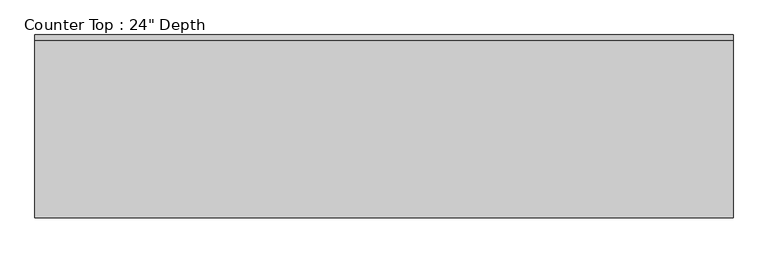
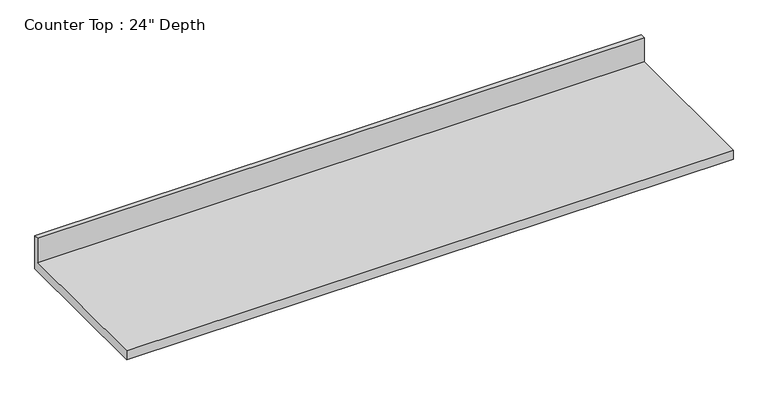
"""IFC4 building model written with IfcOpenShell, lengths in millimetres: furniture geometry."""

from ifc_helpers import new_model, si_unit, frame, origin, place, context, project, spatial, polyline, outline, extrude, source, transform, mapped, element, save


def furniture_bc399e91(model_context):
    return source(origin(), model_context, "Body", "SweptSolid", [
        extrude(outline(polyline([(0.0, 1016.0), (0.0, 876.3), (-635.0, 876.3), (-635.0, 914.4), (-19.05, 914.4), (-19.05, 1016.0), (0.0, 1016.0)])), frame((-1200.4622951, 0.0, 0.0), z_axis=(1.0, 0.0, 0.0), x_axis=(0.0, 1.0, 0.0)), (0.0, 0.0, 1.0), 2425.7),
    ])


if __name__ == "__main__":
    model = new_model("IFC4")
    model_context = context("Model", 3, world=origin())
    ifc_project = project(units=[si_unit("LENGTHUNIT", "METRE", prefix="MILLI")], contexts=[model_context])
    site = spatial("IfcSite", under=ifc_project)
    building = spatial("IfcBuilding", under=site)
    placement = place(None, origin())
    furniture_shape = furniture_bc399e91(model_context)
    element("IfcFurniture", 1, ObjectType="Counter Top : 24\" Depth", at=placement, inside=building, context=model_context, shape_type="MappedRepresentation", body=[
        mapped(furniture_shape, transform((0.0, 0.0, 0.0), x_axis=(1.0, 0.0, 0.0), y_axis=(0.0, 1.0, 0.0), z_axis=(0.0, 0.0, 1.0))),
    ])
    save(model, "model.ifc")

# Revit data of these elements
# Type "Counter Top : 24\" Depth"
#   Assembly Code = "C1030400"
#   Counter Thickness = 0' - 1 1/2"
#   Depth = 2' - 1"
#   Height = 3' - 0"
#   Length [instance default] = 8' - 0"
#   Counter Top Material = none
#   Default Elevation = 0
# Element 1 (IfcFurniture, "Counter Top : 24\" Depth")
#   Length = 7' - 11 1/2"
#   Materials on its faces: "Counter Top"
# Materials
#   "Counter Top": class "Wood", colour RGB 226 177 128, transparency 0
